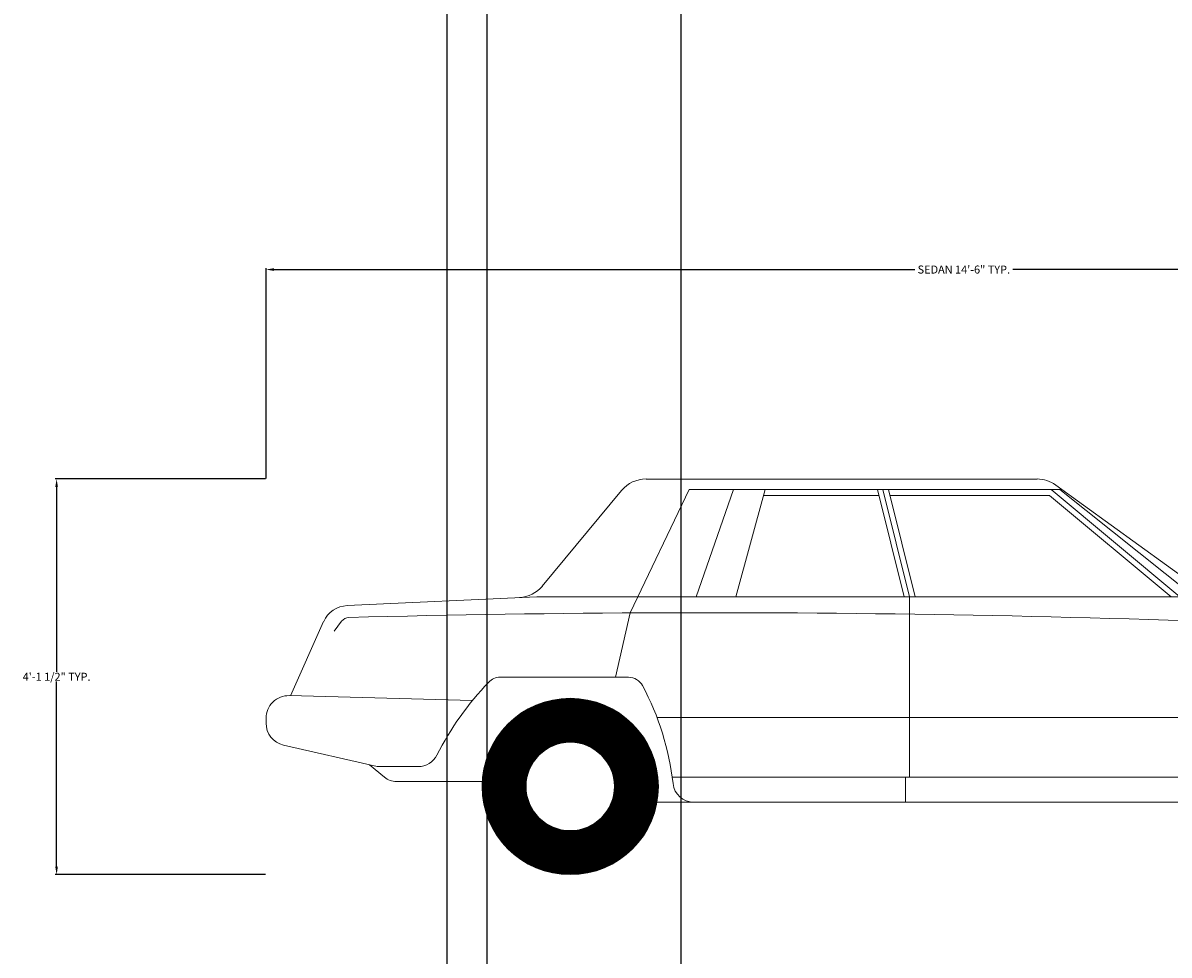
# Model space of a CAD drawing. Units: inches. Extents: x 371 to 1095, y -45 to 1219.
# Tile 6 of 18: x 809 to 952, y 304 to 421. Entities that reach past the tile are written whole.
import ezdxf

# ---------------------------------------------------------------- set-up
doc = ezdxf.new("R2010")
doc.units = ezdxf.units.IN
doc.header["$MEASUREMENT"] = 0
doc.layers.add('A-ANNO-DIMS', color=2, linetype='Continuous', lineweight=18)
doc.layers.add('C-SITE-VEHC', color=8, linetype='Continuous', lineweight=18)
doc.styles.get("Standard").update_dxf_attribs({"font": 'arial.ttf'})
doc.dimstyles.get("Standard").update_dxf_attribs({"dimtxt": 1, "dimasz": 1, "dimexe": 0.18, "dimexo": 0.0625, "dimgap": 0.09, "dimtad": 0, "dimtih": 1, "dimtoh": 1, "dimdec": 0, "dimzin": 0, "dimdsep": 46, "dimlunit": 3, "dimtxsty": 'Standard', "dimcen": 0.09, "dimadec": 0, "dimazin": 0, "dimtfac": 1, "dimtdec": 0, "dimtofl": 0, "dimtmove": 0, "dimatfit": 3, "dimfxl": 1, "dimtolj": 1, "dimtzin": 0, "dimarcsym": 0})

# ---------------------------------------------------------------- blocks, each defined once
blk = doc.blocks.new('Car - sedan  side')
for p, q in [((-77.81, 49.34), (-126.58, 49.34)), ((-139.53, 35.99), (-129.64, 47.91)), ((-128.57, 32.64), (-121.22, 48.02)), ((-74.7, 48.02), (-121.22, 48.02)), ((-120.32, 34.67), (-115.67, 48.02)), ((-115.4, 34.67), (-111.74, 48.02)), ((-97.55, 47.3), (-111.94, 47.3)), ((-94.41, 34.67), (-97.73, 48.02)), ((-93.72, 34.67), (-97.04, 48.02)), ((-93.03, 34.67), (-96.34, 48.02)), ((-76.26, 47.3), (-96.16, 47.3)), ((-61.08, 34.66), (-76.26, 47.3)), ((-60.02, 34.65), (-76.07, 48.02)), ((-56.87, 35.13), (-75.48, 48.59)), ((-58.54, 34.93), (-74.99, 48.02)), ((-140.23, 34.67), (-163.88, 33.56)), ((-62.28, 34.67), (-140.23, 34.67)), ((-93.72, 19.62), (-93.72, 34.67)), ((-62.28, 34.67), (-60.02, 34.65)), ((-170.93, 22.32), (-166.81, 31.56)), ((-164.57, 31.6), (-165.48, 30.35)), ((-130.39, 24.63), (-128.57, 32.64)), ((-128.78, 24.63), (-144.79, 24.63)), ((-148.26, 21.7), (-171.11, 22.33)), ((-174, 19.51), (-174, 18.91)), ((-47.2, 19.62), (-125.23, 19.62)), ((-93.72, 12.14), (-93.72, 19.62)), ((-160.12, 13.48), (-171.81, 16.16)), ((-159.22, 12.14), (-161.08, 13.7)), ((-155.01, 13.48), (-160.12, 13.48)), ((-147.03, 11.6), (-157.73, 11.6)), ((-50.67, 12.14), (-123.32, 12.14)), ((-94.21, 9.03), (-94.21, 12.14)), ((-120.62, 9.03), (-125.23, 9.03)), ((-45.76, 9.03), (-120.62, 9.03))]:
    blk.add_line(p, q)
at = {"const_width": 5.49}
blk.add_lwpolyline([(-127.8, 11, -1), (-144.3, 11, -1)], format="xyb", close=True, dxfattribs=at)
for radius in [11, 5.51]:
    blk.add_circle((-136.05, 11), radius)
for centre, radius, start, end in [((-126.58, 45.38), 3.97, 90, 140.3029), ((-77.81, 45.38), 3.97, 54.135, 90), ((-142.58, 38.53), 3.97, 272.6827, 320.3029), ((-163.72, 30.18), 3.38, 92.6827, 155.9736), ((-163.62, 30.91), 1.17, 91.491, 143.9553), ((-118.51, -1702.12), 1734.79, 86.34698, 91.49105), ((-144.79, 22.64), 1.98, 90, 136.3964), ((-128.78, 22.64), 1.98, 28.1371, 90), ((-118.09, -2.78), 38.85, 136.3964, 152.9097), ((-157.14, 7.48), 34.14, 6.5135, 28.1371), ((-171.18, 19.51), 2.82, 88.4193, 180), ((-171.18, 18.91), 2.82, 180, 257.0905), ((-155.01, 16.1), 2.62, 270, 332.9097), ((-157.73, 13.93), 2.32, 230.1291, 270), ((-120.62, 11.65), 2.62, 186.5135, 270)]:
    blk.add_arc(centre, radius, start, end)
blk = doc.blocks.new('*D38')
at = {"layer": 'A-ANNO-DIMS', "color": 0, "lineweight": -2, "transparency": 16777216}
for p, q in [((839.26, 363.91), (839.26, 390.15)), ((840.26, 389.97), (920.19, 389.97)), ((1012.37, 389.97), (932.44, 389.97)), ((1013.37, 363.91), (1013.37, 390.15))]:
    blk.add_line(p, q, dxfattribs=at)
at = {"layer": 'A-ANNO-DIMS', "color": 0, "transparency": 16777216}
for points in [[(840.26, 390.13), (840.26, 389.8), (839.26, 389.97)], [(1012.37, 390.13), (1012.37, 389.8), (1013.37, 389.97)]]:
    blk.add_solid(points, dxfattribs=at)
at = {"layer": 'Defpoints', "color": 0, "transparency": 16777216}
for p in [(1013.37, 389.97), (839.26, 363.85), (1013.37, 363.85)]:
    blk.add_point(p, dxfattribs=at)
at = {"layer": 'A-ANNO-DIMS', "color": 0, "transparency": 16777216, "insert": (926.31, 389.97), "char_height": 1, "attachment_point": 5}
blk.add_mtext('\\A1;SEDAN 14\'-6" TYP.', dxfattribs=at)
blk = doc.blocks.new('*D39')
at = {"layer": 'A-ANNO-DIMS', "color": 0, "lineweight": -2, "transparency": 16777216}
for p, q in [((839.19, 363.85), (812.96, 363.85)), ((813.14, 362.85), (813.14, 339.78)), ((813.14, 315.5), (813.14, 338.57)), ((839.19, 314.5), (812.96, 314.5))]:
    blk.add_line(p, q, dxfattribs=at)
at = {"layer": 'A-ANNO-DIMS', "color": 0, "transparency": 16777216}
for points in [[(812.97, 362.85), (813.3, 362.85), (813.14, 363.85)], [(812.97, 315.5), (813.3, 315.5), (813.14, 314.5)]]:
    blk.add_solid(points, dxfattribs=at)
at = {"layer": 'Defpoints', "color": 0, "transparency": 16777216}
for p in [(813.14, 363.85), (839.26, 363.85), (839.26, 314.5)]:
    blk.add_point(p, dxfattribs=at)
at = {"layer": 'A-ANNO-DIMS', "color": 0, "transparency": 16777216, "insert": (813.14, 339.18), "char_height": 1, "attachment_point": 5}
blk.add_mtext('\\A1;4\'-1 1/2" TYP.', dxfattribs=at)
blk = doc.blocks.new('*D60')
at = {"layer": 'A-ANNO-DIMS', "color": 0, "lineweight": -2, "transparency": 16777216}
for p, q in [((866.81, 441.96), (866.81, -43.83)), ((891.01, 441.96), (891.01, -43.83)), ((867.81, -43.65), (877.48, -43.65)), ((890.01, -43.65), (880.33, -43.65))]:
    blk.add_line(p, q, dxfattribs=at)
at = {"layer": 'A-ANNO-DIMS', "color": 0, "transparency": 16777216}
for points in [[(867.81, -43.48), (867.81, -43.82), (866.81, -43.65)], [(890.01, -43.48), (890.01, -43.82), (891.01, -43.65)]]:
    blk.add_solid(points, dxfattribs=at)
at = {"layer": 'Defpoints', "color": 0, "transparency": 16777216}
for p in [(866.81, 442.03), (891.01, 442.03), (891.01, -43.65)]:
    blk.add_point(p, dxfattribs=at)
at = {"layer": 'A-ANNO-DIMS', "color": 0, "transparency": 16777216, "insert": (878.91, -43.65), "char_height": 1, "attachment_point": 5}
blk.add_mtext('\\A1;2\'-0"', dxfattribs=at)
blk = doc.blocks.new('*D61')
at = {"layer": 'A-ANNO-DIMS', "color": 0, "lineweight": -2, "transparency": 16777216}
for p, q in [((861.81, 450.96), (861.81, -43.83)), ((866.81, 450.96), (866.81, -43.83)), ((860.81, -43.65), (859.81, -43.65)), ((867.81, -43.65), (868.81, -43.65))]:
    blk.add_line(p, q, dxfattribs=at)
at = {"layer": 'A-ANNO-DIMS', "color": 0, "transparency": 16777216}
for points in [[(860.81, -43.48), (860.81, -43.82), (861.81, -43.65)], [(867.81, -43.48), (867.81, -43.82), (866.81, -43.65)]]:
    blk.add_solid(points, dxfattribs=at)
at = {"layer": 'Defpoints', "color": 0, "transparency": 16777216}
for p in [(861.81, 451.03), (866.81, 451.03), (866.81, -43.65)]:
    blk.add_point(p, dxfattribs=at)
at = {"layer": 'A-ANNO-DIMS', "color": 0, "transparency": 16777216, "insert": (864.31, -43.65), "char_height": 1, "attachment_point": 5}
blk.add_mtext('\\A1;0\'-5"', dxfattribs=at)

msp = doc.modelspace()

# ---------------------------------------------------------------- block references
at = {"layer": 'C-SITE-VEHC'}
msp.add_blockref('Car - sedan  side', (1013.26, 314.5), dxfattribs=at)

# ---------------------------------------------------------------- dimensions: what is measured, and where the dimension line sits
at = {"layer": 'A-ANNO-DIMS'}
for base, p1, p2, picture, middle in [((866.81, -43.65), (861.81, 451.03), (866.81, 451.03), '*D61', (864.31, -43.65)), ((891.01, -43.65), (866.81, 442.03), (891.01, 442.03), '*D60', (878.91, -43.65))]:
    dim = msp.add_linear_dim(base=base, p1=p1, p2=p2, dimstyle='Standard', override={"dimdec": 1, "dimlfac": 1, "dimrnd": 0, "dimzin": 1, "dimdsep": 46, "dimlunit": 4, "dimfrac": 2}, dxfattribs=at)
    dim.commit()
    dim.dimension.update_dxf_attribs({"geometry": picture, "text_midpoint": middle})
dim = msp.add_linear_dim(base=(1013.37, 389.97), p1=(839.26, 363.85), p2=(1013.37, 363.85), text='SEDAN <> TYP.', dimstyle='Standard', override={"dimdec": 1, "dimlfac": 1, "dimrnd": 0, "dimzin": 1, "dimdsep": 46, "dimlunit": 4, "dimfrac": 2}, dxfattribs=at)
dim.commit()
dim.dimension.update_dxf_attribs({"geometry": '*D38', "text_midpoint": (926.31, 389.97)})
dim = msp.add_linear_dim(base=(813.1381, 363.8488), p1=(839.2551, 314.5039), p2=(839.2551, 363.8488), angle=90, text='<> TYP.', dimstyle='Standard', override={"dimdec": 1, "dimlfac": 1, "dimrnd": 0, "dimzin": 1, "dimdsep": 46, "dimlunit": 4, "dimfrac": 2}, dxfattribs=at)
dim.commit()
dim.dimension.update_dxf_attribs({"geometry": '*D39', "text_midpoint": (813.1381, 339.1763)})

doc.saveas('drawing.dxf')
